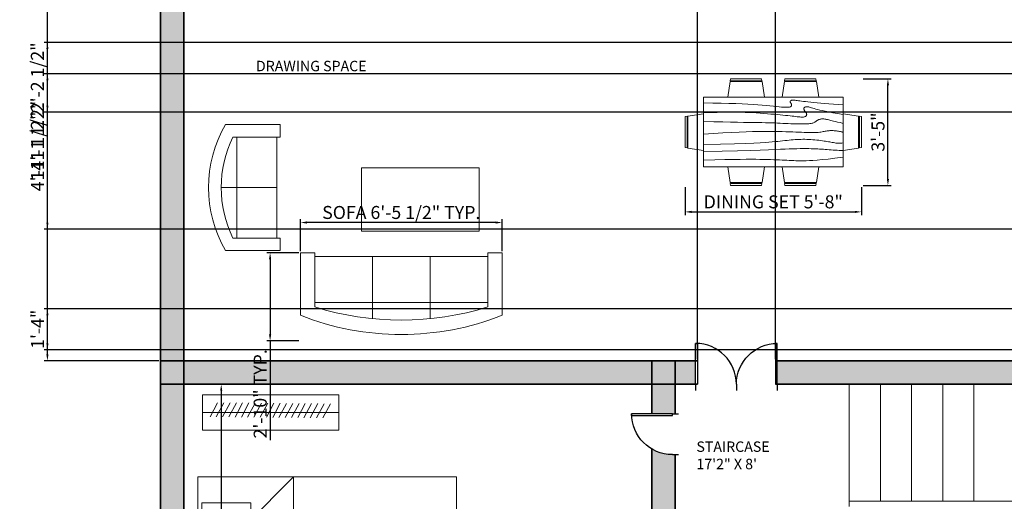
# Model space of a CAD drawing. Units: millimetres. Extents: x 2936 to 3516, y 349 to 1320.
# Tile 2 of 5: x 2936 to 3315, y 763 to 948. Entities that reach past the tile are written whole.
import ezdxf

# ---------------------------------------------------------------- set-up
doc = ezdxf.new("R2010")
doc.units = ezdxf.units.MM
for name, color, linetype, lineweight in [('A-ANNO-DIMS', 3, 'Continuous', 13), ('A-AREA-IDEN', 190, 'Continuous', 18), ('A-FLOR-CASE', 140, 'Continuous', 18), ('A-FLOR-CASE-PATT', 140, 'Continuous', 13), ('A-WALL-PATT', 50, 'Continuous', 13), ('doors', 10, 'Continuous', 25), ('furniture', 140, 'Continuous', 18), ('staircase', 170, 'Continuous', 18), ('walls', 50, 'Continuous', 35)]:
    doc.layers.add(name, color=color, linetype=linetype, lineweight=lineweight)
doc.styles.get("Standard").update_dxf_attribs({"font": 'arial.ttf'})
doc.dimstyles.new('ISO-25', dxfattribs={"dimtxt": 5, "dimasz": 2.5, "dimexe": 1.25, "dimexo": 0.625, "dimtad": 1, "dimdec": 0, "dimlunit": 3, "dimtxsty": 'Standard', "dimcen": 2.5, "dimadec": 0, "dimazin": 0, "dimtfac": 1, "dimtdec": 0, "dimtmove": 0, "dimatfit": 3, "dimfxl": 1, "dimarcsym": 0})

# ---------------------------------------------------------------- blocks, each defined once
blk = doc.blocks.new('*U2')
for p, q in [((0, 0), (0, -6)), ((40, 0), (40, -6))]:
    blk.add_line(p, q)
blk.add_lwpolyline([(0, 0), (0, 40), (1.75, 40), (1.75, 0)], close=True)
blk.add_arc((0, 0), 40, 0, 90)
blk = doc.blocks.new('Sofa - Roundback 7 ft.')
for p, q in [((-12.00002, -32.4421), (-12.00003, -6.5971)), ((11.99997, -32.4421), (11.99998, -6.5971)), ((-36.000027, -34), (-36.000027, -11.4696)), ((35.99998, -34), (35.99998, -11.4696)), ((-35.999844, -13.3819), (35.9998, -13.3819)), ((-36.000027, -32.4421), (35.99998, -32.4421))]:
    blk.add_line(p, q)
for points in [[(-36.000027, -34), (-42.000027, -34), (-42.000027, -8)], [(41.99998, -8), (41.99998, -34), (35.99998, -34)]]:
    blk.add_lwpolyline(points)
for centre, radius, start, end in [((0, -114.25), 114.25, 68.43141, 111.5686), ((-0.00001, -127.1968), 121.1968, 72.72033, 107.2797)]:
    blk.add_arc(centre, radius, start, end)
blk = doc.blocks.new('Sofa - Roundback Loveseat 5 ft.')
for p, q in [((0, -32.44198), (0, -5.99998)), ((-24, -33.99998), (-24, -11.46958)), ((-23.9998, -13.38178), (23.99986, -13.38178)), ((24.00004, -33.99998), (24.00004, -11.46958)), ((-24, -32.44198), (24.00004, -32.44198))]:
    blk.add_line(p, q)
for points in [[(-24, -33.99998), (-30, -33.99998), (-30, -7.99998)], [(30.00004, -7.99998), (30.00004, -33.99998), (24.00004, -33.99998)]]:
    blk.add_lwpolyline(points)
for centre, radius, start, end in [((0, -60.24998), 60.24998, 60.13715, 119.8628), ((0, -61.38438), 55.38444, 64.32083, 115.6792)]:
    blk.add_arc(centre, radius, start, end)
blk = doc.blocks.new('Dining Set - 36 x 72 in.')
for p, q in [((-22.2343, 26.00059), (-23.4847, 17.99762)), ((-22.2304, 26), (-5.7608, 26)), ((-22, 27.5), (-22.1562, 26.50042)), ((-5.8416, 26.5), (-22.1534, 26.5)), ((-22, 27.5), (-6, 27.5)), ((-5.8437, 26.49966), (-6, 27.5)), ((-4.5152, 17.99762), (-5.7655, 25.99926)), ((5.7657, 26.00059), (4.5153, 17.99762)), ((5.7696, 26), (22.2392, 26)), ((6, 27.5), (5.8438, 26.50042)), ((22.1584, 26.5), (5.8466, 26.5)), ((6, 27.5), (22, 27.5)), ((22.1563, 26.49966), (22, 27.5)), ((23.4848, 17.99762), (22.2345, 25.99926)), ((36, 18), (-36, 18)), ((-36, 18), (-36, -18)), ((36, -18), (36, 18)), ((-45.5, 8), (-44.5004, 8.15617)), ((-45.5, 8), (-45.5, -8)), ((-44.5, -8.15843), (-44.5, 8.15338)), ((-44.0006, 8.23428), (-35.9976, 9.48474)), ((-44, 8.23041), (-44, -8.23915)), ((44.0006, 8.23428), (35.9976, 9.48474)), ((44, 8.23041), (44, -8.23915)), ((44.5, -8.15843), (44.5, 8.15338)), ((45.5, 8), (44.5005, 8.15617)), ((45.5, 8), (45.5, -8)), ((-44.4997, -8.15631), (-45.5, -8)), ((-35.9976, -9.48476), (-43.9993, -8.2345)), ((35.9976, -9.48476), (43.9993, -8.2345)), ((44.4997, -8.15631), (45.5, -8)), ((-36, -18), (36, -18)), ((-22.2343, -26.0006), (-23.4847, -17.99762)), ((-4.5152, -17.99762), (-5.7655, -25.99928)), ((5.7657, -26.0006), (4.5153, -17.99762)), ((23.4848, -17.99762), (22.2345, -25.99928)), ((-22.2304, -26), (-5.7608, -26)), ((-22, -27.5), (-22.1562, -26.50044)), ((-5.8416, -26.5), (-22.1534, -26.5)), ((-22, -27.5), (-6, -27.5)), ((-5.8437, -26.49967), (-6, -27.5)), ((5.7696, -26), (22.2392, -26)), ((6, -27.5), (5.8438, -26.50044)), ((22.1584, -26.5), (5.8466, -26.5)), ((6, -27.5), (22, -27.5)), ((22.1563, -26.49967), (22, -27.5))]:
    blk.add_line(p, q)
for points in [[(-36, 15), (-31.1772, 14.97754), (-26.8079, 14.91406), (-22.8538, 14.81543), (-19.276, 14.6875), (-16.0362, 14.53613), (-13.0957, 14.36718), (-10.4159, 14.18652), (-7.9583, 14), (-5.6904, 13.81315), (-3.6035, 13.63021), (-1.6954, 13.45508), (0.0365, 13.29166), (1.5945, 13.14388), (2.9811, 13.01562), (4.1988, 12.9108), (5.25, 12.83333), (6.1393, 12.78613), (6.8802, 12.76823), (7.4883, 12.77767), (7.9792, 12.8125), (8.3685, 12.87077), (8.6719, 12.95052), (8.9049, 13.0498), (9.0833, 13.16666), (9.2205, 13.29899), (9.3216, 13.44401), (9.3895, 13.59879), (9.4271, 13.76041), (9.4373, 13.92594), (9.4232, 14.09245), (9.3875, 14.257), (9.3333, 14.41666), (9.2638, 14.56917), (9.1836, 14.71484), (9.0975, 14.85465), (9.0104, 14.98958), (8.9272, 15.1206), (8.8529, 15.2487), (8.7922, 15.37483), (8.75, 15.5), (8.7305, 15.62467), (8.7344, 15.74739), (8.7617, 15.86621), (8.8125, 15.97916), (8.8867, 16.08431), (8.9844, 16.17968), (9.1055, 16.26334), (9.25, 16.33333), (9.4189, 16.38802), (9.6172, 16.42708), (9.8506, 16.45052), (10.125, 16.45833), (10.4463, 16.45052), (10.8203, 16.42708), (11.2529, 16.38802), (11.75, 16.33333), (12.3184, 16.26318), (12.9694, 16.17838), (13.7151, 16.07991), (14.5677, 15.96875), (15.5395, 15.84586), (16.6426, 15.71224), (17.8893, 15.56884), (19.2917, 15.41666), (20.859, 15.25667), (22.5879, 15.08984), (24.4721, 14.91715), (26.5052, 14.73958), (28.6809, 14.5581), (30.9929, 14.3737), (33.4347, 14.18733), (36, 14)], [(-36, 10), (-28.9766, 10.14274), (-23.1725, 10.20442), (-18.4241, 10.19775), (-14.5677, 10.13541), (-11.4399, 10.03011), (-8.877, 9.89453), (-6.7154, 9.74137), (-4.7917, 9.58333), (-2.9698, 9.43082), (-1.2246, 9.28515), (0.4415, 9.14534), (2.026, 9.01041), (3.5266, 8.87939), (4.9408, 8.7513), (6.266, 8.62516), (7.5, 8.5), (8.6411, 8.37549), (9.6914, 8.2539), (10.6538, 8.13818), (11.5312, 8.03125), (12.3267, 7.93603), (13.043, 7.85547), (13.6831, 7.79248), (14.25, 7.75), (14.7471, 7.7303), (15.1797, 7.73307), (15.5537, 7.75732), (15.875, 7.80208), (16.1494, 7.86637), (16.3828, 7.94922), (16.5811, 8.04964), (16.75, 8.16666), (16.8944, 8.29915), (17.0143, 8.44531), (17.1089, 8.60319), (17.1771, 8.77083), (17.218, 8.94629), (17.2305, 9.1276), (17.2137, 9.31282), (17.1667, 9.5), (17.0895, 9.6875), (16.987, 9.875), (16.8649, 10.0625), (16.7292, 10.25), (16.5856, 10.4375), (16.4401, 10.625), (16.2985, 10.8125), (16.1667, 11), (16.05, 11.18733), (15.9518, 11.3737), (15.8752, 11.5581), (15.8229, 11.73958), (15.798, 11.91715), (15.8034, 12.08984), (15.842, 12.25667), (15.9167, 12.41666), (16.0295, 12.56836), (16.1784, 12.70833), (16.3605, 12.83268), (16.5729, 12.9375), (16.8127, 13.01888), (17.0768, 13.07291), (17.3625, 13.0957), (17.6667, 13.08333), (17.9894, 13.03312), (18.3418, 12.94726), (18.7382, 12.82918), (19.1927, 12.68229), (19.7195, 12.51001), (20.3327, 12.31575), (21.0465, 12.10294), (21.875, 11.875), (22.8357, 11.63354), (23.959, 11.37304), (25.2786, 11.08618), (26.8282, 10.76562), (28.6414, 10.40405), (30.752, 9.99414), (33.1936, 9.52856), (36, 9)], [(-36, 5.5), (-30.7157, 5.3348), (-26.069, 5.20963), (-21.9946, 5.11767), (-18.4271, 5.05208), (-15.3009, 5.00602), (-12.5508, 4.97265), (-10.1112, 4.94515), (-7.9167, 4.91666), (-5.909, 4.88167), (-4.0586, 4.83984), (-2.3429, 4.79215), (-0.7396, 4.73958), (0.7739, 4.6831), (2.22, 4.6237), (3.6213, 4.56233), (5, 4.5), (6.373, 4.43782), (7.7344, 4.3776), (9.0723, 4.32129), (10.375, 4.27083), (11.6309, 4.22819), (12.8281, 4.19531), (13.9551, 4.17415), (15, 4.16666), (15.954, 4.17448), (16.819, 4.19791), (17.6001, 4.23698), (18.3021, 4.29166), (18.9299, 4.36198), (19.4883, 4.44791), (19.9823, 4.54948), (20.4167, 4.66666), (20.7969, 4.79899), (21.1302, 4.94401), (21.4245, 5.09879), (21.6875, 5.26041), (21.9271, 5.42594), (22.1511, 5.59245), (22.3672, 5.757), (22.5834, 5.91666), (22.8065, 6.06868), (23.0404, 6.21093), (23.2879, 6.34147), (23.5521, 6.45833), (23.8358, 6.55957), (24.142, 6.64323), (24.4735, 6.70735), (24.8334, 6.75), (25.2235, 6.76969), (25.642, 6.76692), (26.0858, 6.74267), (26.5521, 6.69791), (27.0379, 6.63362), (27.5404, 6.55078), (28.0565, 6.45036), (28.5834, 6.33333), (29.1242, 6.19987), (29.7071, 6.04687), (30.3661, 5.87044), (31.1354, 5.66666), (32.0493, 5.43164), (33.142, 5.16146), (34.4475, 4.85221), (36, 4.5)], [(-36, -1), (-30.7915, -0.6591), (-26.0195, -0.38216), (-21.6519, -0.16284), (-17.6563, 0.00521), (-14.0005, 0.12833), (-10.6523, 0.21289), (-7.5796, 0.26522), (-4.75, 0.29166), (-2.134, 0.29793), (0.2878, 0.28711), (2.5317, 0.26163), (4.6146, 0.22396), (6.5529, 0.17651), (8.3633, 0.12174), (10.0623, 0.06209), (11.6667, 0), (13.1899, -0.06201), (14.6341, -0.1211), (15.9982, -0.17432), (17.2813, -0.21875), (18.4823, -0.25147), (19.6003, -0.26953), (20.6343, -0.27002), (21.5834, -0.25), (22.4481, -0.20768), (23.2357, -0.14584), (23.9549, -0.06836), (24.6146, 0.02083), (25.2235, 0.11784), (25.7904, 0.21875), (26.3241, 0.31966), (26.8334, 0.41666), (27.3265, 0.50618), (27.8099, 0.58593), (28.2894, 0.65397), (28.7709, 0.70833), (29.2601, 0.74707), (29.763, 0.76823), (30.2855, 0.76985), (30.8334, 0.75), (31.4088, 0.70784), (31.9994, 0.64713), (32.589, 0.57275), (33.1615, 0.48958), (33.7008, 0.4025), (34.1908, 0.3164), (34.6153, 0.23616), (34.9584, 0.16666), (35.2099, 0.11165), (35.3848, 0.07031), (35.504, 0.04069), (35.5886, 0.02083), (35.6594, 0.00879), (35.7377, 0.0026), (35.8442, 0.00032), (36, 0)], [(-36, -6.5), (-27.1843, -6.31267), (-20.084, -6.1263), (-14.469, -5.9419), (-10.1094, -5.76042), (-6.7752, -5.58285), (-4.2363, -5.41016), (-2.2629, -5.24333), (-0.625, -5.08334), (0.8708, -4.93099), (2.2715, -4.78646), (3.5872, -4.64974), (4.8281, -4.52084), (6.0046, -4.39974), (7.127, -4.28646), (8.2053, -4.18099), (9.25, -4.08334), (10.2705, -3.99382), (11.2734, -3.91407), (12.2647, -3.84603), (13.25, -3.79167), (14.2354, -3.75293), (15.2266, -3.73177), (16.2295, -3.73015), (17.25, -3.75), (18.2912, -3.79248), (19.3451, -3.85547), (20.4009, -3.93604), (21.4479, -4.03125), (22.4754, -4.13819), (23.4727, -4.25391), (24.4289, -4.37549), (25.3334, -4.5), (26.1785, -4.62492), (26.9694, -4.74935), (27.7145, -4.87281), (28.4219, -4.99479), (29.1, -5.11483), (29.7572, -5.23242), (30.4016, -5.34709), (31.0417, -5.45834), (31.6837, -5.56437), (32.3262, -5.65821), (32.9658, -5.73153), (33.599, -5.77604), (34.2224, -5.78345), (34.8327, -5.74545), (35.4264, -5.65373), (36, -5.5)], [(-36, -10), (-26.4022, -9.81299), (-18.4675, -9.62891), (-11.9839, -9.45069), (-6.7396, -9.28125), (-2.5226, -9.12354), (0.8789, -8.98047), (3.6769, -8.85498), (6.0833, -8.75), (8.2767, -8.66765), (10.3021, -8.60677), (12.1712, -8.56543), (13.8958, -8.54167), (15.4876, -8.53353), (16.9583, -8.53907), (18.3197, -8.55632), (19.5834, -8.58334), (20.7616, -8.61841), (21.8685, -8.66081), (22.9188, -8.71004), (23.9271, -8.76563), (24.9081, -8.82707), (25.8763, -8.89388), (26.8465, -8.96558), (27.8334, -9.04167), (28.8474, -9.12118), (29.8828, -9.20117), (30.93, -9.27824), (31.9792, -9.34896), (33.0205, -9.40991), (34.0443, -9.45768), (35.0407, -9.48885), (36, -9.5)], [(-36, -14.5), (-30.0881, -14.33513), (-25.0332, -14.21224), (-20.7312, -14.12647), (-17.0781, -14.07292), (-13.97, -14.04671), (-11.3027, -14.04297), (-8.9724, -14.05681), (-6.875, -14.08334), (-4.9224, -14.11833), (-3.0905, -14.16016), (-1.3709, -14.20785), (0.2448, -14.26042), (1.7647, -14.3169), (3.1973, -14.3763), (4.5507, -14.43767), (5.8333, -14.5), (7.0554, -14.5621), (8.235, -14.62175), (9.3922, -14.67652), (10.5469, -14.72396), (11.7192, -14.76164), (12.929, -14.78711), (14.1965, -14.79794), (15.5417, -14.79167), (16.9933, -14.76424), (18.6152, -14.70508), (20.4804, -14.60197), (22.6615, -14.44271), (25.2312, -14.21509), (28.2624, -13.9069), (31.8277, -13.50594), (36, -13)]]:
    blk.add_lwpolyline(points)
blk = doc.blocks.new('Bed - Queen')
for p, q in [((0, -80.00003), (0, 0)), ((0, 0), (59.99999, 0)), ((59.99999, 0), (59.99999, -80.00003)), ((7.99999, -1.2), (28.79998, -1.2)), ((7.99999, -14.4), (7.99999, -1.2)), ((28.79998, -1.2), (28.79998, -14.4)), ((31.19999, -1.2), (51.99999, -1.2)), ((31.19999, -14.4), (31.19999, -1.2)), ((51.99999, -1.2), (51.99999, -16.4)), ((0, -14.4), (44.8, -14.4)), ((59.99999, -29.6), (44.8, -14.4)), ((44.8, -14.4), (44.8, -29.6)), ((44.8, -16.8), (0, -16.8)), ((51.99999, -16.4), (46.79936, -16.4)), ((44.8, -29.6), (59.99999, -29.6)), ((59.99999, -80.00003), (0, -80.00003))]:
    blk.add_line(p, q)
blk = doc.blocks.new('*D28')
at = {"layer": 'A-ANNO-DIMS', "color": 0, "lineweight": -2, "transparency": 16777216}
for p, q in [((3003.81, 807.86), (3014.77, 807.86)), ((3013.52, 805.36), (3013.52, 686.36)), ((3003.81, 683.86), (3014.77, 683.86))]:
    blk.add_line(p, q, dxfattribs=at)
at = {"layer": 'A-ANNO-DIMS', "color": 0, "transparency": 16777216}
for points in [[(3013.11, 805.36), (3013.94, 805.36), (3013.52, 807.86)], [(3013.11, 686.36), (3013.94, 686.36), (3013.52, 683.86)]]:
    blk.add_solid(points, dxfattribs=at)
at = {"layer": 'Defpoints', "color": 0, "transparency": 16777216}
for p in [(3003.19, 807.86), (3003.19, 683.86), (3013.52, 683.86)]:
    blk.add_point(p, dxfattribs=at)
at = {"layer": 'A-ANNO-DIMS', "color": 0, "transparency": 16777216, "insert": (3010.34, 745.86), "char_height": 5, "attachment_point": 5, "rotation": 90}
blk.add_mtext('10\'-4"', dxfattribs=at)
blk = doc.blocks.new('COFFEE-TABLE-RECT')
blk.add_lwpolyline([(0, 24.44), (45.27, 24.44), (45.27, 0), (0, 0)], close=True)
blk = doc.blocks.new('*D45')
at = {"layer": 'A-ANNO-DIMS', "color": 0, "lineweight": -2, "transparency": 16777216}
for p, q in [((3043.99, 859.05), (3043.99, 871.32)), ((3119.13, 870.07), (3046.49, 870.07)), ((3121.63, 859.05), (3121.63, 871.32))]:
    blk.add_line(p, q, dxfattribs=at)
at = {"layer": 'A-ANNO-DIMS', "color": 0, "transparency": 16777216}
for points in [[(3046.49, 870.49), (3046.49, 869.66), (3043.99, 870.07)], [(3119.13, 870.49), (3119.13, 869.66), (3121.63, 870.07)]]:
    blk.add_solid(points, dxfattribs=at)
at = {"layer": 'Defpoints', "color": 0, "transparency": 16777216}
for p in [(3043.99, 870.07), (3043.99, 858.43), (3121.63, 858.43)]:
    blk.add_point(p, dxfattribs=at)
at = {"layer": 'A-ANNO-DIMS', "color": 0, "transparency": 16777216, "insert": (3082.81, 873.29), "char_height": 5, "attachment_point": 5}
blk.add_mtext('SOFA 6\'-5 1/2" TYP.', dxfattribs=at)
blk = doc.blocks.new('*D46')
at = {"layer": 'A-ANNO-DIMS', "color": 0, "lineweight": -2, "transparency": 16777216}
for p, q in [((3043.36, 858.43), (3031.09, 858.43)), ((3032.34, 855.93), (3032.34, 827.03)), ((3043.36, 824.53), (3031.09, 824.53)), ((3032.34, 824.53), (3032.34, 786.33))]:
    blk.add_line(p, q, dxfattribs=at)
at = {"layer": 'A-ANNO-DIMS', "color": 0, "transparency": 16777216}
for points in [[(3031.92, 855.93), (3032.75, 855.93), (3032.34, 858.43)], [(3031.92, 827.03), (3032.75, 827.03), (3032.34, 824.53)]]:
    blk.add_solid(points, dxfattribs=at)
at = {"layer": 'Defpoints', "color": 0, "transparency": 16777216}
for p in [(3043.99, 858.43), (3032.34, 824.53), (3043.99, 824.53)]:
    blk.add_point(p, dxfattribs=at)
at = {"layer": 'A-ANNO-DIMS', "color": 0, "transparency": 16777216, "insert": (3029.16, 804.18), "char_height": 5, "attachment_point": 5, "rotation": 90}
blk.add_mtext('2\'-10" TYP.', dxfattribs=at)
blk = doc.blocks.new('*D51')
at = {"layer": 'A-ANNO-DIMS', "color": 0, "lineweight": -2, "transparency": 16777216}
for p, q in [((3192.02, 883.72), (3192.02, 872.91)), ((3259.89, 883.72), (3259.89, 872.91)), ((3194.52, 874.16), (3257.39, 874.16))]:
    blk.add_line(p, q, dxfattribs=at)
at = {"layer": 'A-ANNO-DIMS', "color": 0, "transparency": 16777216}
for points in [[(3194.52, 874.58), (3194.52, 873.75), (3192.02, 874.16)], [(3257.39, 874.58), (3257.39, 873.75), (3259.89, 874.16)]]:
    blk.add_solid(points, dxfattribs=at)
at = {"layer": 'Defpoints', "color": 0, "transparency": 16777216}
for p in [(3192.02, 884.34), (3259.89, 884.34), (3259.89, 874.16)]:
    blk.add_point(p, dxfattribs=at)
at = {"layer": 'A-ANNO-DIMS', "color": 0, "transparency": 16777216, "insert": (3225.96, 877.37), "char_height": 5, "attachment_point": 5}
blk.add_mtext('DINING SET 5\'-8"', dxfattribs=at)
blk = doc.blocks.new('*D52')
at = {"layer": 'A-ANNO-DIMS', "color": 0, "lineweight": -2, "transparency": 16777216}
for p, q in [((3260.52, 925.37), (3271.32, 925.37)), ((3270.07, 886.84), (3270.07, 922.87)), ((3260.52, 884.34), (3271.32, 884.34))]:
    blk.add_line(p, q, dxfattribs=at)
at = {"layer": 'A-ANNO-DIMS', "color": 0, "transparency": 16777216}
for points in [[(3269.66, 922.87), (3270.49, 922.87), (3270.07, 925.37)], [(3269.66, 886.84), (3270.49, 886.84), (3270.07, 884.34)]]:
    blk.add_solid(points, dxfattribs=at)
at = {"layer": 'Defpoints', "color": 0, "transparency": 16777216}
for p in [(3259.89, 925.37), (3270.07, 925.37), (3259.89, 884.34)]:
    blk.add_point(p, dxfattribs=at)
at = {"layer": 'A-ANNO-DIMS', "color": 0, "transparency": 16777216, "insert": (3266.9, 904.86), "char_height": 5, "attachment_point": 5, "rotation": 90}
blk.add_mtext('3\'-5"', dxfattribs=at)
blk = doc.blocks.new('*D57')
at = {"layer": 'A-ANNO-DIMS', "color": 0, "lineweight": -2, "transparency": 16777216}
for p, q in [((2989.57, 986.28), (2945.39, 986.28)), ((2946.64, 819.36), (2946.64, 983.78)), ((2989.57, 816.86), (2945.39, 816.86))]:
    blk.add_line(p, q, dxfattribs=at)
at = {"layer": 'A-ANNO-DIMS', "color": 0, "transparency": 16777216}
for points in [[(2946.22, 983.78), (2947.06, 983.78), (2946.64, 986.28)], [(2946.22, 819.36), (2947.06, 819.36), (2946.64, 816.86)]]:
    blk.add_solid(points, dxfattribs=at)
at = {"layer": 'Defpoints', "color": 0, "transparency": 16777216}
for p in [(2946.64, 986.28), (2990.19, 986.28), (2990.19, 816.86)]:
    blk.add_point(p, dxfattribs=at)
at = {"layer": 'A-ANNO-DIMS', "color": 0, "transparency": 16777216, "insert": (2943.43, 901.57), "char_height": 5, "attachment_point": 5, "rotation": 90}
blk.add_mtext('14\'-1 1/2"', dxfattribs=at)
blk = doc.blocks.new('*D60')
at = {"layer": 'A-ANNO-DIMS', "color": 0, "lineweight": -2, "transparency": 16777216}
for p, q in [((3320.57, 927.28), (2945.39, 927.28)), ((2946.64, 870.06), (2946.64, 924.78)), ((3320.57, 867.56), (2945.39, 867.56))]:
    blk.add_line(p, q, dxfattribs=at)
at = {"layer": 'A-ANNO-DIMS', "color": 0, "transparency": 16777216}
for points in [[(2946.22, 924.78), (2947.06, 924.78), (2946.64, 927.28)], [(2946.22, 870.06), (2947.06, 870.06), (2946.64, 867.56)]]:
    blk.add_solid(points, dxfattribs=at)
at = {"layer": 'Defpoints', "color": 0, "transparency": 16777216}
for p in [(2946.64, 927.28), (3321.19, 927.28), (3321.19, 867.56)]:
    blk.add_point(p, dxfattribs=at)
at = {"layer": 'A-ANNO-DIMS', "color": 0, "transparency": 16777216, "insert": (2943.43, 897.42), "char_height": 5, "attachment_point": 5, "rotation": 90}
blk.add_mtext('4\'-11 1/2"', dxfattribs=at)
blk = doc.blocks.new('*D62')
at = {"layer": 'A-ANNO-DIMS', "color": 0, "lineweight": -2, "transparency": 16777216}
for p, q in [((3359.43, 836.89), (2945.39, 836.89)), ((2946.64, 823.63), (2946.64, 834.39)), ((3359.43, 821.13), (2945.39, 821.13))]:
    blk.add_line(p, q, dxfattribs=at)
at = {"layer": 'A-ANNO-DIMS', "color": 0, "transparency": 16777216}
for points in [[(2946.22, 834.39), (2947.06, 834.39), (2946.64, 836.89)], [(2946.22, 823.63), (2947.06, 823.63), (2946.64, 821.13)]]:
    blk.add_solid(points, dxfattribs=at)
at = {"layer": 'Defpoints', "color": 0, "transparency": 16777216}
for p in [(2946.64, 836.89), (3360.06, 836.89), (3360.06, 821.13)]:
    blk.add_point(p, dxfattribs=at)
at = {"layer": 'A-ANNO-DIMS', "color": 0, "transparency": 16777216, "insert": (2943.51, 829.01), "char_height": 5, "attachment_point": 5, "rotation": 90}
blk.add_mtext('1\'-4"', dxfattribs=at)
blk = doc.blocks.new('*D64')
at = {"layer": 'A-ANNO-DIMS', "color": 0, "lineweight": -2, "transparency": 16777216}
for p, q in [((3441.54, 939.3), (2945.39, 939.3)), ((2946.64, 915.06), (2946.64, 936.8)), ((3441.54, 912.56), (2945.39, 912.56))]:
    blk.add_line(p, q, dxfattribs=at)
at = {"layer": 'A-ANNO-DIMS', "color": 0, "transparency": 16777216}
for points in [[(2946.22, 936.8), (2947.06, 936.8), (2946.64, 939.3)], [(2946.22, 915.06), (2947.06, 915.06), (2946.64, 912.56)]]:
    blk.add_solid(points, dxfattribs=at)
at = {"layer": 'Defpoints', "color": 0, "transparency": 16777216}
for p in [(2946.64, 939.3), (3442.16, 939.3), (3442.16, 912.56)]:
    blk.add_point(p, dxfattribs=at)
at = {"layer": 'A-ANNO-DIMS', "color": 0, "transparency": 16777216, "insert": (2943.43, 925.93), "char_height": 5, "attachment_point": 5, "rotation": 90}
blk.add_mtext('2\'-2 1/2"', dxfattribs=at)
blk = doc.blocks.new('*D66')
at = {"layer": 'A-ANNO-DIMS', "color": 0, "lineweight": -2, "transparency": 16777216}
for p, q in [((3196.76, 817.48), (3196.76, 1310.08)), ((3199.26, 1308.83), (3224.31, 1308.83)), ((3226.81, 817.48), (3226.81, 1310.08))]:
    blk.add_line(p, q, dxfattribs=at)
at = {"layer": 'A-ANNO-DIMS', "color": 0, "transparency": 16777216}
for points in [[(3199.26, 1309.25), (3199.26, 1308.42), (3196.76, 1308.83)], [(3224.31, 1309.25), (3224.31, 1308.42), (3226.81, 1308.83)]]:
    blk.add_solid(points, dxfattribs=at)
at = {"layer": 'Defpoints', "color": 0, "transparency": 16777216}
for p in [(3226.81, 1308.83), (3196.76, 816.86), (3226.81, 816.86)]:
    blk.add_point(p, dxfattribs=at)
at = {"layer": 'A-ANNO-DIMS', "color": 0, "transparency": 16777216, "insert": (3211.79, 1312.01), "char_height": 5, "attachment_point": 5}
blk.add_mtext('2\'-6"', dxfattribs=at)

msp = doc.modelspace()

# ---------------------------------------------------------------- hatches: boundary and pattern name
at = {"layer": 'A-FLOR-CASE-PATT'}
h = msp.add_hatch(dxfattribs=at)
h.set_pattern_fill('ANSI31', color=256, scale=0.672729, angle=16.819, style=0)
h.paths.add_polyline_path([(3007.7, 795.38), (3053.5, 794.94), (3056.41, 800.36), (3010.6, 800.8)])
at = {"layer": 'A-WALL-PATT'}
h = msp.add_hatch(color=256, dxfattribs=at)
h.dxf.hatch_style = 1
h.paths.add_polyline_path([(2999.19, 1256.28), (2990.19, 1256.28), (2990.19, 1160.28), (2999.19, 1160.28)])
h.paths.add_polyline_path([(2999.19, 1265.28), (2990.19, 1265.28), (2990.19, 1256.28), (2999.19, 1256.28)])
h.paths.add_polyline_path([(3024.89, 1265.28), (2999.19, 1265.28), (2999.19, 1256.28), (3024.89, 1256.28)])
h.paths.add_polyline_path([(3074.24, 1160.28), (2999.19, 1160.28), (2999.19, 1151.28), (3072.14, 1151.28), (3072.14, 1152.43, -0.131652)])
h.paths.add_polyline_path([(2999.19, 1160.28), (2990.19, 1160.28), (2990.19, 1151.28), (2999.19, 1151.28)])
h.paths.add_polyline_path([(3123.19, 1256.28), (3114.19, 1256.28), (3114.19, 1160.28), (3123.19, 1160.28)])
h.paths.add_polyline_path([(3123.19, 1160.28), (3114.19, 1160.28), (3114.19, 1151.28), (3123.19, 1151.28)])
h.paths.add_polyline_path([(3114.19, 1160.28), (3087.85, 1160.28), (3087.85, 1152.43), (3087.85, 1151.28), (3114.19, 1151.28)])
h.paths.add_polyline_path([(3114.19, 1265.28), (3068.72, 1265.28), (3068.72, 1256.28), (3114.19, 1256.28)])
h.paths.add_polyline_path([(3123.19, 1265.28), (3114.19, 1265.28), (3114.19, 1256.28), (3123.19, 1256.28)])
h.paths.add_polyline_path([(3143.16, 1265.28), (3123.19, 1265.28), (3123.19, 1256.28), (3143.16, 1256.28)])
h.paths.add_polyline_path([(3214.19, 1265.28), (3187.49, 1265.28), (3187.49, 1256.28), (3214.19, 1256.28)])
h.paths.add_polyline_path([(3214.19, 1160.28), (3140.09, 1160.28, -0.121149), (3141.88, 1153), (3141.88, 1151.28), (3214.19, 1151.28)])
h.paths.add_polyline_path([(3223.19, 1256.28), (3214.19, 1256.28), (3214.19, 1160.28), (3223.19, 1160.28)])
h.paths.add_polyline_path([(3223.19, 1160.28), (3214.19, 1160.28), (3214.19, 1151.28), (3223.19, 1151.28)])
h.paths.add_polyline_path([(3223.19, 1151.28), (3214.19, 1151.28), (3214.19, 1134.28), (3223.19, 1134.28)])
h.paths.add_polyline_path([(3223.19, 1134.28), (3214.19, 1134.28), (3214.19, 1125.28), (3223.19, 1125.28)])
h.paths.add_polyline_path([(3223.19, 1125.28), (3214.19, 1125.28), (3214.19, 1064.28), (3223.19, 1064.28)])
h.paths.add_polyline_path([(3281.06, 1126.52, -0.130008), (3283.12, 1134.28), (3223.19, 1134.28), (3223.19, 1125.28), (3281.06, 1125.28)])
h.paths.add_polyline_path([(3223.19, 1265.28), (3214.19, 1265.28), (3214.19, 1256.28), (3223.19, 1256.28)])
h.paths.add_polyline_path([(3235.61, 1265.28), (3223.19, 1265.28), (3223.19, 1256.28), (3235.61, 1256.28)])
h.paths.add_polyline_path([(3297.19, 1265.28), (3278.85, 1265.28), (3278.85, 1256.28), (3297.19, 1256.28)])
h.paths.add_polyline_path([(3306.19, 1265.28), (3297.19, 1265.28), (3297.19, 1256.28), (3306.19, 1256.28)])
h.paths.add_polyline_path([(3306.19, 1256.28), (3297.19, 1256.28), (3297.19, 1134.28), (3306.19, 1134.28)])
h.paths.add_polyline_path([(3306.19, 1134.28), (3297.19, 1134.28), (3297.19, 1125.28), (3306.19, 1125.28)])
h.paths.add_polyline_path([(3306.19, 1125.28), (3297.19, 1125.28), (3297.19, 1084.87), (3305.61, 1084.87), (3306.19, 1084.87)])
h.paths.add_polyline_path([(3365.17, 1265.28), (3306.19, 1265.28), (3306.19, 1256.28), (3365.17, 1256.28)])
h.paths.add_polyline_path([(3462.19, 1265.28), (3409.24, 1265.28), (3409.24, 1256.28), (3462.19, 1256.28)])
h.paths.add_polyline_path([(3471.19, 1265.28), (3462.19, 1265.28), (3462.19, 1256.28), (3471.19, 1256.28)])
h.paths.add_polyline_path([(3471.19, 1256.28), (3462.19, 1256.28), (3462.19, 1225.41), (3471.19, 1225.41)])
h.paths.add_polyline_path([(3471.19, 1177.19), (3462.19, 1177.19), (3462.19, 1064.28), (3471.19, 1064.28)])
h.paths.add_polyline_path([(3462.19, 1064.28), (3368.33, 1064.28), (3368.33, 1055.28), (3462.19, 1055.28)])
h.paths.add_polyline_path([(3471.19, 1064.28), (3462.19, 1064.28), (3462.19, 1055.28), (3471.19, 1055.28)])
h.paths.add_polyline_path([(3471.19, 1055.28), (3462.19, 1055.28), (3462.19, 969.86), (3471.19, 969.86)])
h.paths.add_polyline_path([(3368.33, 1055.28), (3359.33, 1055.28), (3359.33, 995.28), (3368.33, 995.28)])
h.paths.add_polyline_path([(3368.33, 1064.28), (3359.33, 1064.28), (3359.33, 1055.28), (3368.33, 1055.28)])
h.paths.add_polyline_path([(3359.33, 995.28), (3306.19, 995.28), (3306.19, 986.28), (3359.33, 986.28)])
h.paths.add_polyline_path([(3368.33, 995.28), (3359.33, 995.28), (3359.33, 986.28), (3368.33, 986.28)])
h.paths.add_polyline_path([(3306.19, 995.28), (3297.19, 995.28), (3297.19, 986.28), (3306.19, 986.28)])
h.paths.add_polyline_path([(3306.19, 1011.04), (3298.85, 1011.04), (3297.19, 1011.04), (3297.19, 995.28), (3306.19, 995.28)])
h.paths.add_polyline_path([(3306.19, 1055.28), (3297.19, 1055.28), (3297.19, 1026.75), (3298.85, 1026.75, -0.122211), (3306.19, 1024.93)])
h.paths.add_polyline_path([(3306.19, 1064.28), (3297.19, 1064.28), (3297.19, 1055.28), (3306.19, 1055.28)])
h.paths.add_polyline_path([(3297.19, 1064.28), (3223.19, 1064.28), (3223.19, 1055.28), (3297.19, 1055.28)])
h.paths.add_polyline_path([(3223.19, 1064.28), (3214.19, 1064.28), (3214.19, 1055.28), (3223.19, 1055.28)])
h.paths.add_polyline_path([(3223.19, 1055.28), (3214.19, 1055.28), (3214.19, 1031.96), (3221.18, 1031.96), (3223.19, 1031.96)])
h.paths.add_polyline_path([(3223.19, 1016.25), (3221.18, 1016.25, -0.11578), (3214.19, 1017.89), (3214.19, 995.28), (3223.19, 995.28)])
h.paths.add_polyline_path([(3223.19, 995.28), (3214.19, 995.28), (3214.19, 986.28), (3223.19, 986.28)])
h.paths.add_polyline_path([(3214.19, 995.28), (3061.3, 995.28), (3061.3, 986.28), (3214.19, 986.28)])
h.paths.add_polyline_path([(2999.19, 1151.28), (2990.19, 1151.28), (2990.19, 995.28), (2999.19, 995.28)])
h.paths.add_polyline_path([(2999.19, 986.28), (2990.19, 986.28), (2990.19, 816.86), (2999.19, 816.86)])
h.paths.add_polyline_path([(2999.19, 995.28), (2990.19, 995.28), (2990.19, 986.28), (2999.19, 986.28)])
h.paths.add_polyline_path([(3016.23, 995.28), (2999.19, 995.28), (2999.19, 986.28), (3016.23, 986.28)])
h.paths.add_polyline_path([(2999.19, 807.86), (2990.19, 807.86), (2990.19, 683.86), (2999.19, 683.86)])
h.paths.add_polyline_path([(2999.19, 816.86), (2990.19, 816.86), (2990.19, 807.86), (2999.19, 807.86)])
h.paths.add_polyline_path([(3179.19, 816.86), (2999.19, 816.86), (2999.19, 807.86), (3179.19, 807.86)])
h.paths.add_polyline_path([(3188.19, 780.83), (3187.16, 780.83, -0.133677), (3179.19, 783), (3179.19, 683.86), (3188.19, 683.86)])
h.paths.add_polyline_path([(3188.19, 807.86), (3179.19, 807.86), (3179.19, 796.54), (3187.16, 796.54), (3188.19, 796.54)])
h.paths.add_polyline_path([(3188.19, 816.86), (3179.19, 816.86), (3179.19, 807.86), (3188.19, 807.86)])
h.paths.add_polyline_path([(3196.08, 816.86), (3188.19, 816.86), (3188.19, 807.86), (3196.08, 807.86)])
h.paths.add_polyline_path([(3321.19, 816.86), (3227.5, 816.86), (3227.5, 807.86), (3321.19, 807.86)])
h.paths.add_polyline_path([(3330.19, 867.56), (3321.19, 867.56), (3321.19, 816.86), (3330.19, 816.86)])
h.paths.add_polyline_path([(3330.19, 816.86), (3321.19, 816.86), (3321.19, 807.86), (3330.19, 807.86)])
h.paths.add_polyline_path([(3462.19, 816.86), (3330.19, 816.86), (3330.19, 807.86), (3462.19, 807.86)])
h.paths.add_polyline_path([(3471.19, 960.86), (3462.19, 960.86), (3462.19, 816.86), (3471.19, 816.86)])
h.paths.add_polyline_path([(3471.19, 816.86), (3462.19, 816.86), (3462.19, 807.86), (3471.19, 807.86)])
h.paths.add_polyline_path([(3471.19, 807.86), (3462.19, 807.86), (3462.19, 394.29), (3471.19, 394.29)])
h.paths.add_polyline_path([(3462.19, 715.94), (3227.5, 715.94), (3227.5, 708.13), (3227.5, 706.94), (3462.19, 706.94)])
h.paths.add_polyline_path([(3196.08, 715.94), (3188.19, 715.94), (3188.19, 706.94), (3196.08, 706.94), (3196.08, 708.13)])
h.paths.add_polyline_path([(2999.19, 674.86), (2990.19, 674.86), (2990.19, 554.86), (2999.19, 554.86)])
h.paths.add_polyline_path([(3179.19, 683.86), (2999.19, 683.86), (2999.19, 674.86), (3179.19, 674.86)])
h.paths.add_polyline_path([(2999.19, 683.86), (2990.19, 683.86), (2990.19, 674.86), (2999.19, 674.86)])
h.paths.add_polyline_path([(2999.19, 545.86), (2990.19, 545.86), (2990.19, 394.29), (2999.19, 394.29)])
h.paths.add_polyline_path([(3047.58, 554.86), (2999.19, 554.86), (2999.19, 545.86), (3047.58, 545.86)])
h.paths.add_polyline_path([(2999.19, 554.86), (2990.19, 554.86), (2990.19, 545.86), (2999.19, 545.86)])
h.paths.add_polyline_path([(3179.19, 554.86), (3096.19, 554.86), (3096.19, 545.86), (3179.19, 545.86)])
h.paths.add_polyline_path([(3188.19, 554.86), (3179.19, 554.86), (3179.19, 545.86), (3188.19, 545.86)])
h.paths.add_polyline_path([(3188.19, 652.99), (3187.11, 652.99, -0.132871), (3179.19, 655.13), (3179.19, 554.86), (3188.19, 554.86)])
h.paths.add_polyline_path([(3188.19, 683.86), (3179.19, 683.86), (3179.19, 674.86), (3188.19, 674.86)])
h.paths.add_polyline_path([(3188.19, 674.86), (3179.19, 674.86), (3179.19, 668.7), (3187.11, 668.7), (3188.19, 668.7)])
h.paths.add_polyline_path([(3462.19, 969.86), (3330.19, 969.86), (3330.19, 960.86), (3462.19, 960.86)])
h.paths.add_polyline_path([(3330.19, 969.86), (3321.19, 969.86), (3321.19, 960.86), (3330.19, 960.86)])
h.paths.add_polyline_path([(3330.19, 960.86), (3321.19, 960.86), (3321.19, 927.28), (3330.19, 927.28)])

# ---------------------------------------------------------------- linework, layer by layer
at = {"layer": 'A-FLOR-CASE'}
msp.add_line((3006.35, 796.97), (3058.72, 796.97), dxfattribs=at)
msp.add_lwpolyline([(3006.35, 803.79), (3058.72, 803.79), (3058.72, 790.15), (3006.35, 790.15)], close=True, dxfattribs=at)
at = {"layer": 'staircase'}
for p, q in [((3255.17, 807.86), (3255.17, 762.86)), ((3267.17, 807.86), (3267.17, 762.86)), ((3279.17, 807.86), (3279.17, 762.86)), ((3291.17, 807.86), (3291.17, 762.86)), ((3303.17, 807.86), (3303.17, 762.86)), ((3423.17, 762.86), (3255.17, 762.86)), ((3255.17, 762.86), (3255.17, 762.86)), ((3255.17, 762.86), (3255.17, 760.86))]:
    msp.add_line(p, q, dxfattribs=at)
at = {"layer": 'walls'}
for p, q in [((2990.19, 1265.28), (2990.19, 394.29)), ((2999.19, 1265.28), (2999.19, 394.29)), ((3196.76, 816.86), (2990.19, 816.86)), ((3179.19, 816.86), (3179.19, 796.54)), ((3188.19, 816.86), (3188.19, 796.54)), ((3471.19, 816.86), (3226.81, 816.86)), ((3196.76, 807.86), (2990.19, 807.86)), ((3471.19, 807.86), (3226.81, 807.86)), ((3179.19, 783), (3179.19, 668.7)), ((3188.19, 780.83), (3188.19, 668.7))]:
    msp.add_line(p, q, dxfattribs=at)

# ---------------------------------------------------------------- block references
at = {"layer": 'doors', "yscale": 0.3927729305520136, "zscale": 0.3927729305520136}
for p, xscale, rotation in [((3196.08, 807.86), 0.3927729305520136, 1.02022929505e-05), ((3227.5, 807.86), -0.3927729305520136, 359.9999897977093), ((3187.16, 796.54), -0.3927729305520136, 90)]:
    msp.add_blockref('*U2', p, dxfattribs=dict(at, xscale=xscale, rotation=rotation))
at = {"layer": 'furniture', "xscale": 0.7458529914065825, "yscale": 0.7458529914065825, "zscale": 0.7458529914065825}
msp.add_blockref('Dining Set - 36 x 72 in.', (3225.96, 904.86), dxfattribs=at)
at = {"layer": 'furniture'}
for name, p, xscale, yscale, zscale, rotation in [('Sofa - Roundback Loveseat 5 ft.', (3008.67, 883.52), 0.8087673324917968, 0.8087673324917968, 0.8087673324917968, 90), ('Sofa - Roundback 7 ft.', (3082.81, 827), 0.9243959546179767, 0.9243959546179767, 0.9243959546179767, 180), ('Bed - Queen', (3004.51, 697.53), 1.245124643961403, 1.245124643961403, 1.245124643961403, 90)]:
    msp.add_blockref(name, p, dxfattribs=dict(at, xscale=xscale, yscale=yscale, zscale=zscale, rotation=rotation))
msp.add_blockref('COFFEE-TABLE-RECT', (3067.56, 866.7), dxfattribs=at)

# ---------------------------------------------------------------- texts
at = {"layer": 'A-AREA-IDEN', "char_height": 4, "attachment_point": 1}
for s, width, insert in [('DRAWING SPACE', 57.502, (3026.89, 932.26)), ('STAIRCASE\\P17\'2" X 8\'', 53.4137, (3196.39, 785.87))]:
    msp.add_mtext_dynamic_manual_height_columns(s, width=width, gutter_width=12.5, heights=[0], dxfattribs=dict(at, insert=insert))

# ---------------------------------------------------------------- dimensions: what is measured, and where the dimension line sits
at = {"layer": 'A-ANNO-DIMS'}
dim = msp.add_linear_dim(base=(3226.8118, 1308.8345), p1=(3196.7646, 816.8556), p2=(3226.8118, 816.8556), dimstyle='ISO-25', override={"dimdec": 1, "dimlfac": 1, "dimrnd": 0, "dimzin": 1, "dimdsep": 46, "dimlunit": 4, "dimfrac": 2}, dxfattribs=at)
dim.commit()
dim.dimension.update_dxf_attribs({"geometry": '*D66', "text_midpoint": (3211.7882, 1312.0124)})
for base, p1, p2, override, picture, middle in [((2946.64, 986.28), (2990.19, 816.86), (2990.19, 986.28), {"dimdec": 1, "dimlfac": 1, "dimrnd": 0, "dimzin": 1, "dimdsep": 46, "dimlunit": 4, "dimfrac": 2}, '*D57', (2943.43, 901.57)), ((2946.64, 939.3), (3442.16, 912.56), (3442.16, 939.3), {"dimdec": 1, "dimlfac": 1, "dimrnd": 0, "dimzin": 1, "dimdsep": 46, "dimlunit": 4, "dimfrac": 2}, '*D64', (2943.43, 925.93)), ((2946.64, 927.28), (3321.19, 867.56), (3321.19, 927.28), {"dimdec": 1, "dimlfac": 1, "dimrnd": 0, "dimzin": 1, "dimdsep": 46, "dimlunit": 4, "dimfrac": 2}, '*D60', (2943.43, 897.42)), ((3270.07, 925.37), (3259.89, 884.34), (3259.89, 925.37), {"dimdec": 1, "dimlfac": 1, "dimrnd": 0, "dimzin": 1, "dimdsep": 46, "dimlunit": 4, "dimfrac": 2}, '*D52', (3266.9, 904.86)), ((2946.64, 836.89), (3360.06, 821.13), (3360.06, 836.89), {"dimdec": 1, "dimlfac": 1, "dimrnd": 0, "dimzin": 1, "dimdsep": 46, "dimlunit": 4, "dimfrac": 2}, '*D62', (2943.51, 829.01)), ((3013.52, 683.86), (3003.19, 807.86), (3003.19, 683.86), {"dimclrd": 0, "dimclre": 0, "dimclrt": 0}, '*D28', (3010.34, 745.86))]:
    dim = msp.add_linear_dim(base=base, p1=p1, p2=p2, angle=90, dimstyle='ISO-25', override=override, dxfattribs=at)
    dim.commit()
    dim.dimension.update_dxf_attribs({"geometry": picture, "text_midpoint": middle})
for base, p1, p2, angle, text, picture, middle in [((3043.99, 870.07), (3121.63, 858.43), (3043.99, 858.43), 180, 'SOFA <> TYP.', '*D45', (3082.81, 873.29)), ((3032.34, 824.53), (3043.99, 858.43), (3043.99, 824.53), 270, '<> TYP.', '*D46', (3029.16, 804.18))]:
    dim = msp.add_linear_dim(base=base, p1=p1, p2=p2, angle=angle, text=text, dimstyle='ISO-25', override={"dimdec": 1, "dimlfac": 1, "dimrnd": 0, "dimzin": 1, "dimdsep": 46, "dimlunit": 4, "dimfrac": 2}, dxfattribs=at)
    dim.commit()
    dim.dimension.update_dxf_attribs({"geometry": picture, "text_midpoint": middle})
dim = msp.add_linear_dim(base=(3259.89, 874.16), p1=(3192.02, 884.34), p2=(3259.89, 884.34), text='DINING SET <>', dimstyle='ISO-25', override={"dimdec": 1, "dimlfac": 1, "dimrnd": 0, "dimzin": 1, "dimdsep": 46, "dimlunit": 4, "dimfrac": 2}, dxfattribs=at)
dim.commit()
dim.dimension.update_dxf_attribs({"geometry": '*D51', "text_midpoint": (3225.96, 877.37)})

doc.saveas('drawing.dxf')
